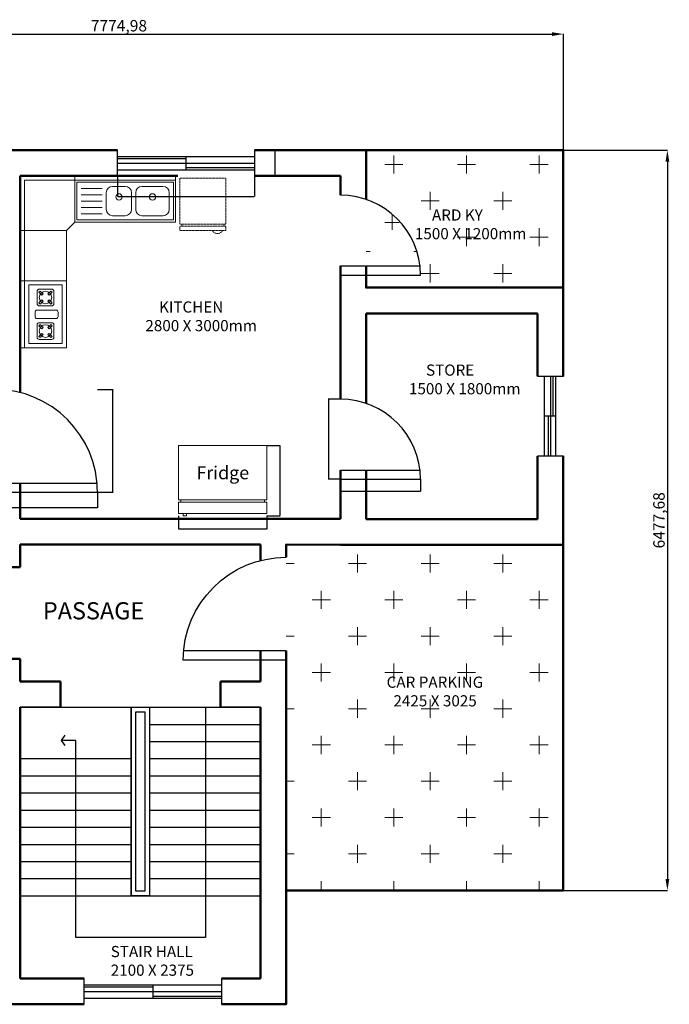
# Model space of a CAD drawing. Units: millimetres. Extents: x -857 to 54106, y -13666 to 13947.
# Tile 12 of 41: x 11637 to 17319, y 5329 to 13947. Entities that reach past the tile are written whole.
import ezdxf

# ---------------------------------------------------------------- set-up
doc = ezdxf.new("R2010")
doc.units = ezdxf.units.MM
doc.linetypes.add('HIDDEN', pattern=[0.375, 0.25, -0.125])
for name, color, linetype, lineweight in [('A-ANNO-DIMS', 2, 'Continuous', 18), ('A-AREA-IDEN', 3, 'Continuous', 18), ('A-DOOR', 1, 'Continuous', 25), ('A-FLOR-FIXT', 8, 'Continuous', 18), ('A-FLOR-FIXT-OVHD', 8, 'HIDDEN', 18), ('A-FLOR-PATT', 252, 'Continuous', 13), ('A-FLOR-STRS', 30, 'Continuous', 25), ('A-GLAZ', 4, 'Continuous', 25), ('A-WALL', 7, 'Continuous', 50), ('FURNITURE', 25, 'Continuous', 9)]:
    doc.layers.add(name, color=color, linetype=linetype, lineweight=lineweight)
doc.styles.add('k.k.', font='arial.ttf')
doc.styles.get("Standard").update_dxf_attribs({"font": 'arial.ttf'})
doc.dimstyles.new('ISO-25', dxfattribs={"dimtxt": 2.5, "dimasz": 2.5, "dimexe": 1.25, "dimexo": 0.625, "dimtad": 1, "dimtxsty": 'Standard', "dimcen": 2.5, "dimadec": 0, "dimazin": 0, "dimtfac": 1, "dimtmove": 0, "dimatfit": 3, "dimfxl": 1, "dimarcsym": 0})

# ---------------------------------------------------------------- blocks, each defined once
blk = doc.blocks.new('A$C338378D9')
at = {"layer": 'FURNITURE'}
for p, q in [((1, -25), (1, -24)), ((38, -25), (38, -24))]:
    blk.add_line(p, q, dxfattribs=at)
for points in [[(0, -24), (39, -24), (39, 0), (0, 0)], [(0, -30), (39, -30), (39, -25), (0, -25)], [(3.5, -31), (2, -31), (2, -30), (3.5, -30)]]:
    blk.add_lwpolyline(points, close=True, dxfattribs=at)
blk = doc.blocks.new('*D25')
at = {"layer": 'A-ANNO-DIMS', "color": 0, "lineweight": -2, "transparency": 16777216}
for p, q in [((8617.3, 12804.9), (8617.3, 13821.5)), ((8717.3, 13820.3), (16292.3, 13820.3)), ((16392.3, 12804.9), (16392.3, 13821.5))]:
    blk.add_line(p, q, dxfattribs=at)
at = {"layer": 'A-ANNO-DIMS', "color": 0, "transparency": 16777216}
for points in [[(8717.3, 13837), (8717.3, 13803.6), (8617.3, 13820.3)], [(16292.3, 13837), (16292.3, 13803.6), (16392.3, 13820.3)]]:
    blk.add_solid(points, dxfattribs=at)
at = {"layer": 'Defpoints', "color": 0, "transparency": 16777216}
for p in [(16392.3, 13820.3), (8617.3, 12804.2), (16392.3, 12804.2)]:
    blk.add_point(p, dxfattribs=at)
at = {"layer": 'A-ANNO-DIMS', "color": 0, "transparency": 16777216, "insert": (12504.8, 13881), "char_height": 100, "attachment_point": 5}
blk.add_mtext('7774,98', dxfattribs=at)
blk = doc.blocks.new('*D26')
at = {"layer": 'A-ANNO-DIMS', "color": 0, "lineweight": -2, "transparency": 16777216}
for p, q in [((16392.9, 12804.2), (17303.8, 12804.2)), ((17302.5, 12704.2), (17302.5, 6426.6)), ((16392.9, 6326.6), (17303.8, 6326.6))]:
    blk.add_line(p, q, dxfattribs=at)
at = {"layer": 'A-ANNO-DIMS', "color": 0, "transparency": 16777216}
for points in [[(17285.9, 12704.2), (17319.2, 12704.2), (17302.5, 12804.2)], [(17285.9, 6426.6), (17319.2, 6426.6), (17302.5, 6326.6)]]:
    blk.add_solid(points, dxfattribs=at)
at = {"layer": 'Defpoints', "color": 0, "transparency": 16777216}
for p in [(16392.3, 12804.2), (16392.3, 6326.6), (17302.5, 6326.6)]:
    blk.add_point(p, dxfattribs=at)
at = {"layer": 'A-ANNO-DIMS', "color": 0, "transparency": 16777216, "insert": (17241.8, 9565.4), "char_height": 100, "attachment_point": 5, "rotation": 90}
blk.add_mtext('6477,68', dxfattribs=at)
blk = doc.blocks.new('DOOR-900')
blk.add_line((11417.3, 9811.5), (12317.3, 9811.5))
blk.add_arc((11417.3, 9811.5), 900, 0, 90)
blk = doc.blocks.new('DOOR-700')
blk.add_line((8245.5, 10779.2), (8245.5, 11479.2))
blk.add_arc((8245.5, 10779.2), 700, 90, 180)
blk = doc.blocks.new('WIN-1200')
for p, q in [((9371.3, 11750.2), (10571.3, 11750.2)), ((9371.3, 11731.7), (9971.3, 11731.7)), ((9971.3, 11750.2), (9971.3, 11630.7)), ((9371.3, 11691.7), (10571.3, 11691.7)), ((9971.3, 11651.7), (10571.3, 11651.7)), ((10571.3, 11630.7), (9371.3, 11630.7))]:
    blk.add_line(p, q)
for points in [[(9371.3, 11579.2), (9371.3, 11804.2)], [(10571.3, 11804.2), (10571.3, 11579.2)]]:
    blk.add_lwpolyline(points)
blk = doc.blocks.new('WIN-700')
for p, q in [((3626.3, 8304.2), (3626.3, 9004.2)), ((3679.8, 9004.2), (3679.8, 8304.2)), ((3699.8, 9004.2), (3699.8, 8654.2)), ((3724.4, 9004.2), (3724.4, 8304.2)), ((3724.4, 8654.2), (3626.3, 8654.2)), ((3659.8, 8654.2), (3659.8, 8304.2))]:
    blk.add_line(p, q)
for points in [[(3567.3, 9004.2), (3792.3, 9004.2)], [(3792.3, 8304.2), (3567.3, 8304.2)]]:
    blk.add_lwpolyline(points)
blk = doc.blocks.new('*D31')
at = {"layer": 'A-ANNO-DIMS', "color": 0, "lineweight": -2, "transparency": 16777216}
for p, q in [((11417.3, 9810.9), (11417.3, 9675.2)), ((12317.3, 9810.9), (12317.3, 9675.2)), ((11419.8, 9676.5), (12314.8, 9676.5))]:
    blk.add_line(p, q, dxfattribs=at)
at = {"layer": 'A-ANNO-DIMS', "color": 0, "transparency": 16777216}
for points in [[(11419.8, 9676.9), (11419.8, 9676.1), (11417.3, 9676.5)], [(12314.8, 9676.9), (12314.8, 9676.1), (12317.3, 9676.5)]]:
    blk.add_solid(points, dxfattribs=at)
at = {"layer": 'Defpoints', "color": 0, "transparency": 16777216}
for p in [(11417.3, 9811.5), (12317.3, 9811.5), (12317.3, 9676.5)]:
    blk.add_point(p, dxfattribs=at)
at = {"layer": 'A-ANNO-DIMS', "color": 0, "transparency": 16777216, "insert": (11867.3, 9678.4), "char_height": 2.5, "attachment_point": 5}
blk.add_mtext('DOOR D1 900 TYP.', dxfattribs=at)
blk = doc.blocks.new('*D32')
at = {"layer": 'A-ANNO-DIMS', "color": 0, "lineweight": -2, "transparency": 16777216}
for p, q in [((12317.9, 10711.5), (12453.5, 10711.5)), ((12452.3, 9814), (12452.3, 10709)), ((12317.9, 9811.5), (12453.5, 9811.5))]:
    blk.add_line(p, q, dxfattribs=at)
at = {"layer": 'A-ANNO-DIMS', "color": 0, "transparency": 16777216}
for points in [[(12451.9, 10709), (12452.7, 10709), (12452.3, 10711.5)], [(12451.9, 9814), (12452.7, 9814), (12452.3, 9811.5)]]:
    blk.add_solid(points, dxfattribs=at)
at = {"layer": 'Defpoints', "color": 0, "transparency": 16777216}
for p in [(12317.3, 10711.5), (12452.3, 10711.5), (12317.3, 9811.5)]:
    blk.add_point(p, dxfattribs=at)
at = {"layer": 'A-ANNO-DIMS', "color": 0, "transparency": 16777216, "insert": (12450.4, 10261.5), "char_height": 2.5, "attachment_point": 5, "rotation": 90}
blk.add_mtext('900 TYP.', dxfattribs=at)
blk = doc.blocks.new('*D33')
at = {"layer": 'A-ANNO-DIMS', "color": 0, "lineweight": -2, "transparency": 16777216}
for p, q in [((14441.7, 10624.9), (14336, 10624.9)), ((14337.3, 10622.4), (14337.3, 9927.4)), ((14441.7, 9924.9), (14336, 9924.9))]:
    blk.add_line(p, q, dxfattribs=at)
at = {"layer": 'A-ANNO-DIMS', "color": 0, "transparency": 16777216}
for points in [[(14336.9, 10622.4), (14337.7, 10622.4), (14337.3, 10624.9)], [(14336.9, 9927.4), (14337.7, 9927.4), (14337.3, 9924.9)]]:
    blk.add_solid(points, dxfattribs=at)
at = {"layer": 'Defpoints', "color": 0, "transparency": 16777216}
for p in [(14442.3, 10624.9), (14337.3, 9924.9), (14442.3, 9924.9)]:
    blk.add_point(p, dxfattribs=at)
at = {"layer": 'A-ANNO-DIMS', "color": 0, "transparency": 16777216, "insert": (14335.4, 10274.9), "char_height": 2.5, "attachment_point": 5, "rotation": 90}
blk.add_mtext('DOOR D2 700 TYP.', dxfattribs=at)
blk = doc.blocks.new('*D34')
at = {"layer": 'A-ANNO-DIMS', "color": 0, "lineweight": -2, "transparency": 16777216}
for p, q in [((14442.3, 9924.3), (14442.3, 9818.7)), ((15142.3, 9924.3), (15142.3, 9818.7)), ((14444.8, 9819.9), (15139.8, 9819.9))]:
    blk.add_line(p, q, dxfattribs=at)
at = {"layer": 'A-ANNO-DIMS', "color": 0, "transparency": 16777216}
for points in [[(14444.8, 9820.4), (14444.8, 9819.5), (14442.3, 9819.9)], [(15139.8, 9820.4), (15139.8, 9819.5), (15142.3, 9819.9)]]:
    blk.add_solid(points, dxfattribs=at)
at = {"layer": 'Defpoints', "color": 0, "transparency": 16777216}
for p in [(14442.3, 9924.9), (15142.3, 9924.9), (15142.3, 9819.9)]:
    blk.add_point(p, dxfattribs=at)
at = {"layer": 'A-ANNO-DIMS', "color": 0, "transparency": 16777216, "insert": (14792.3, 9821.8), "char_height": 2.5, "attachment_point": 5}
blk.add_mtext('700 TYP.', dxfattribs=at)
blk = doc.blocks.new('*D35')
at = {"layer": 'A-ANNO-DIMS', "color": 0, "lineweight": -2, "transparency": 16777216}
for p, q in [((12491.5, 12578.6), (12491.5, 12398)), ((13691.5, 12578.6), (13691.5, 12398)), ((12494, 12399.2), (13689, 12399.2))]:
    blk.add_line(p, q, dxfattribs=at)
at = {"layer": 'A-ANNO-DIMS', "color": 0, "transparency": 16777216}
for points in [[(12494, 12399.6), (12494, 12398.8), (12491.5, 12399.2)], [(13689, 12399.6), (13689, 12398.8), (13691.5, 12399.2)]]:
    blk.add_solid(points, dxfattribs=at)
at = {"layer": 'Defpoints', "color": 0, "transparency": 16777216}
for p in [(12491.5, 12579.2), (13691.5, 12579.2), (13691.5, 12399.2)]:
    blk.add_point(p, dxfattribs=at)
at = {"layer": 'A-ANNO-DIMS', "color": 0, "transparency": 16777216, "insert": (13091.5, 12401.1), "char_height": 2.5, "attachment_point": 5}
blk.add_mtext('WINDOW W1 1200 TYP.', dxfattribs=at)
blk = doc.blocks.new('*D36')
at = {"layer": 'A-ANNO-DIMS', "color": 0, "lineweight": -2, "transparency": 16777216}
for p, q in [((13692.1, 12804.2), (13872.7, 12804.2)), ((13871.5, 12581.7), (13871.5, 12801.7)), ((13692.1, 12579.2), (13872.7, 12579.2))]:
    blk.add_line(p, q, dxfattribs=at)
at = {"layer": 'A-ANNO-DIMS', "color": 0, "transparency": 16777216}
for points in [[(13871.1, 12801.7), (13871.9, 12801.7), (13871.5, 12804.2)], [(13871.1, 12581.7), (13871.9, 12581.7), (13871.5, 12579.2)]]:
    blk.add_solid(points, dxfattribs=at)
at = {"layer": 'Defpoints', "color": 0, "transparency": 16777216}
for p in [(13691.5, 12804.2), (13871.5, 12804.2), (13691.5, 12579.2)]:
    blk.add_point(p, dxfattribs=at)
at = {"layer": 'A-ANNO-DIMS', "color": 0, "transparency": 16777216, "insert": (13869.6, 12691.7), "char_height": 2.5, "attachment_point": 5, "rotation": 90}
blk.add_mtext('225 TYP.', dxfattribs=at)
blk = doc.blocks.new('*D61')
at = {"layer": 'A-ANNO-DIMS', "color": 0, "lineweight": -2, "transparency": 16777216}
for p, q in [((13026.8, 9604.5), (13026.8, 9488)), ((13799.4, 9604.5), (13799.4, 9488)), ((13029.3, 9489.3), (13796.9, 9489.3))]:
    blk.add_line(p, q, dxfattribs=at)
at = {"layer": 'A-ANNO-DIMS', "color": 0, "transparency": 16777216}
for points in [[(13029.3, 9489.7), (13029.3, 9488.8), (13026.8, 9489.3)], [(13796.9, 9489.7), (13796.9, 9488.8), (13799.4, 9489.3)]]:
    blk.add_solid(points, dxfattribs=at)
at = {"layer": 'Defpoints', "color": 0, "transparency": 16777216}
for p in [(13026.8, 9605.1), (13799.4, 9605.1), (13799.4, 9489.3)]:
    blk.add_point(p, dxfattribs=at)
at = {"layer": 'A-ANNO-DIMS', "color": 0, "transparency": 16777216, "insert": (13413.1, 9491.2), "char_height": 2.5, "attachment_point": 5}
blk.add_mtext('FRIDGE 773', dxfattribs=at)
blk = doc.blocks.new('*D62')
at = {"layer": 'A-ANNO-DIMS', "color": 0, "lineweight": -2, "transparency": 16777216}
for p, q in [((13800, 10219.2), (13916.5, 10219.2)), ((13915.3, 9607.6), (13915.3, 10216.7)), ((13800, 9605.1), (13916.5, 9605.1))]:
    blk.add_line(p, q, dxfattribs=at)
at = {"layer": 'A-ANNO-DIMS', "color": 0, "transparency": 16777216}
for points in [[(13914.8, 10216.7), (13915.7, 10216.7), (13915.3, 10219.2)], [(13914.8, 9607.6), (13915.7, 9607.6), (13915.3, 9605.1)]]:
    blk.add_solid(points, dxfattribs=at)
at = {"layer": 'Defpoints', "color": 0, "transparency": 16777216}
for p in [(13799.4, 10219.2), (13915.3, 10219.2), (13799.4, 9605.1)]:
    blk.add_point(p, dxfattribs=at)
at = {"layer": 'A-ANNO-DIMS', "color": 0, "transparency": 16777216, "insert": (13913.3, 9912.2), "char_height": 2.5, "attachment_point": 5, "rotation": 90}
blk.add_mtext('614', dxfattribs=at)

msp = doc.modelspace()

# ---------------------------------------------------------------- hatches: boundary and pattern name
at = {"layer": 'A-FLOR-PATT'}
h = msp.add_hatch(dxfattribs=at)
h.set_pattern_fill('CROSS', color=256, scale=50)
h.set_pattern_definition([(0, (-5489.92, -2561.3), (317.5, 317.5), [158.75, -476.25]), (90, (-5410.54, -2640.7), (-317.5, 317.5), [158.75, -476.25])])
h.paths.add_polyline_path([(16392.264, 9351.555), (14441.85, 9351.555), (13967.28, 9353.369), (13967.28, 9241.901), (13967.28, 8421.901), (13967.28, 6326.555), (16392.264, 6326.555)])
h.paths.add_polyline_path([(16392.264, 12804.231), (14667.264, 12804.231), (14667.264, 12374.147, -0.32131534), (15142.28, 11711.288), (14667.264, 11711.288), (14667.264, 11601.555), (16392.264, 11601.555)])
h.paths.add_polyline_path([(11417.28, 12804.231), (8617.28, 12804.231), (8617.28, 11804.231), (9371.341, 11804.231), (9371.341, 11750.152), (10571.341, 11750.152), (10571.341, 11804.231), (11417.28, 11804.231)])
h = msp.add_hatch(dxfattribs=at)
h.set_pattern_fill('CROSS', color=256, scale=40)
h.set_pattern_definition([(0, (-5489.92, -2561.3), (254, 254), [127, -381]), (90, (-5426.42, -2624.8), (-254, 254), [127, -381])])
h.paths.add_polyline_path([(14667.264, 12374.147), (14667.264, 11791.288), (15137.693, 11791.288, 0.29000459)])

# ---------------------------------------------------------------- linework, layer by layer
at = {"layer": 'A-DOOR'}
for p, q in [((14442.28, 11791.288), (15142.28, 11791.288)), ((14442.28, 10004.935), (15142.28, 10004.935)), ((11417.28, 9891.481), (12317.28, 9891.481)), ((13967.28, 8421.901), (13067.28, 8421.901))]:
    msp.add_line(p, q, dxfattribs=at)
at = {"layer": 'A-FLOR-FIXT'}
for p, q in [((13000.196, 12542.53), (12119.386, 12542.53)), ((12357.938, 12469.13), (12174.436, 12469.13)), ((12357.938, 12414.079), (12174.436, 12414.079)), ((12357.938, 12414.079), (12174.436, 12414.079)), ((12357.938, 12359.028), (12174.436, 12359.028)), ((12357.938, 12303.978), (12174.436, 12303.978)), ((12357.938, 12248.927), (12174.436, 12248.927)), ((11678.98, 12102.125), (11678.98, 11661.72)), ((11678.98, 11661.72), (11678.98, 11074.513))]:
    msp.add_line(p, q, dxfattribs=at)
for points in [[(12119.386, 12175.526), (12119.386, 12579.231), (11642.28, 12579.231), (11642.28, 12102.125), (12045.985, 12102.125)], [(13000.196, 12175.526), (13000.196, 12579.231), (12119.386, 12579.231), (12119.386, 12175.526)], [(12981.846, 12193.876), (12981.846, 12524.18), (12137.736, 12524.18), (12137.736, 12193.876)], [(12045.985, 12102.125), (11642.28, 12102.125), (11642.28, 11661.72), (12045.985, 11661.72)], [(12045.985, 11661.72), (11642.28, 11661.72), (11642.28, 11074.513), (12045.985, 11074.513)], [(12009.284, 11625.019), (11715.681, 11625.019), (11715.681, 11111.213), (12009.284, 11111.213)], [(11831.341, 11535.679), (11805.39, 11561.63), (11815.771, 11572.011), (11841.722, 11546.06)], [(11893.624, 11535.679), (11919.575, 11561.63), (11909.195, 11572.011), (11883.243, 11546.06)], [(11831.341, 11494.157), (11805.39, 11468.206), (11815.771, 11457.826), (11841.722, 11483.777)], [(11893.624, 11494.157), (11919.575, 11468.206), (11909.195, 11457.826), (11883.243, 11483.777)], [(11831.341, 11242.076), (11805.39, 11268.027), (11815.771, 11278.407), (11841.722, 11252.456)], [(11893.624, 11242.076), (11919.575, 11268.027), (11909.195, 11278.407), (11883.243, 11252.456)], [(11831.341, 11200.554), (11805.39, 11174.603), (11815.771, 11164.222), (11841.722, 11190.173)], [(11893.624, 11200.554), (11919.575, 11174.603), (11909.195, 11164.222), (11883.243, 11190.173)]]:
    msp.add_lwpolyline(points, close=True, dxfattribs=at)
msp.add_lwpolyline([(12119.386, 12542.53), (11678.98, 12542.53), (11678.98, 12102.125)], dxfattribs=at)
for points in [[(12559.791, 12487.48, -0.41421356), (12614.842, 12432.429), (12614.842, 12285.627, -0.41421356), (12559.791, 12230.577), (12449.69, 12230.577, -0.41421356), (12394.639, 12285.627), (12394.639, 12432.429, -0.41421356), (12449.69, 12487.48)], [(12890.095, 12487.48, -0.41421356), (12945.145, 12432.429), (12945.145, 12285.627, -0.41421356), (12890.095, 12230.577), (12706.593, 12230.577, -0.41421356), (12651.542, 12285.627), (12651.542, 12432.429, -0.41421356), (12706.593, 12487.48)], [(11935.883, 11459.868), (11935.883, 11569.969, 0.41421356), (11917.533, 11588.319), (11807.432, 11588.319, 0.41421356), (11789.082, 11569.969), (11789.082, 11459.868, 0.41421356), (11807.432, 11441.517), (11917.533, 11441.517, 0.41421356)], [(11972.584, 11349.766), (11972.584, 11386.467, 0.41421356), (11954.234, 11404.817), (11789.082, 11404.817, 0.41421356), (11770.731, 11386.467), (11770.731, 11349.766, 0.41421356), (11789.082, 11331.416), (11954.234, 11331.416, 0.41421356)], [(11935.883, 11276.365), (11935.883, 11166.264, -0.41421356), (11917.533, 11147.914), (11807.432, 11147.914, -0.41421356), (11789.082, 11166.264), (11789.082, 11276.365, -0.41421356), (11807.432, 11294.716), (11917.533, 11294.716, -0.41421356)]]:
    msp.add_lwpolyline(points, format="xyb", close=True, dxfattribs=at)
for centre, radius in [((12504.74, 12395.729), 27.525), ((12798.344, 12395.729), 27.525), ((11862.483, 11514.918), 55.051), ((11862.483, 11221.315), 55.051)]:
    msp.add_circle(centre, radius, dxfattribs=at)
at = {"layer": 'A-FLOR-FIXT-OVHD'}
for p, q in [((13055.247, 12138.826), (13055.247, 12157.176)), ((13422.251, 12138.826), (13422.251, 12157.176)), ((13440.601, 12138.826), (13036.897, 12138.826)), ((13036.897, 12138.826), (13036.897, 12102.125)), ((13036.897, 12102.125), (13440.601, 12102.125)), ((13440.601, 12102.125), (13440.601, 12138.826))]:
    msp.add_line(p, q, dxfattribs=at)
msp.add_lwpolyline([(13440.601, 12560.881), (13440.601, 12157.176), (13036.897, 12157.176), (13036.897, 12560.881)], close=True, dxfattribs=at)
msp.add_arc((13366.68, 12122.628), 48.348, 205.0922551, 334.9077449, dxfattribs=at)
at = {"layer": 'A-FLOR-STRS'}
for p, q in [((11992.28, 7929.231), (11642.28, 7929.231)), ((11642.28, 7929.231), (13742.28, 7929.231)), ((12612.28, 7929.231), (12612.28, 6279.231)), ((12772.28, 7929.231), (12772.28, 6279.231)), ((13742.28, 7929.231), (13392.28, 7929.231)), ((12772.28, 7779.231), (13742.28, 7779.231)), ((12772.28, 7629.231), (13742.28, 7629.231)), ((11642.28, 7479.231), (12612.28, 7479.231)), ((12772.28, 7479.231), (13742.28, 7479.231)), ((11642.28, 7329.231), (12612.28, 7329.231)), ((12772.28, 7329.231), (13742.28, 7329.231)), ((11642.28, 7179.231), (12612.28, 7179.231)), ((12772.28, 7179.231), (13742.28, 7179.231)), ((11642.28, 7029.231), (12612.28, 7029.231)), ((12772.28, 7029.231), (13742.28, 7029.231)), ((11642.28, 6879.231), (12612.28, 6879.231)), ((12772.28, 6879.231), (13742.28, 6879.231)), ((11642.28, 6729.231), (12612.28, 6729.231)), ((12772.28, 6729.231), (13742.28, 6729.231)), ((11642.28, 6579.231), (12612.28, 6579.231)), ((12772.28, 6579.231), (13742.28, 6579.231)), ((11642.28, 6429.231), (12612.28, 6429.231)), ((12772.28, 6429.231), (13742.28, 6429.231)), ((11642.28, 6279.231), (13742.28, 6279.231))]:
    msp.add_line(p, q, dxfattribs=at)
for points in [[(13263.236, 7929.231), (13263.236, 5914.255), (12127.28, 5914.255), (12127.28, 7637.854), (12000.518, 7637.854)], [(12031.972, 7684.139), (12000.518, 7637.854), (12030.82, 7594.913)]]:
    msp.add_lwpolyline(points, dxfattribs=at)
for points in [[(12612.28, 7929.231), (12772.28, 7929.231), (12772.28, 6279.231), (12612.28, 6279.231)], [(12652.28, 7889.231), (12732.28, 7889.231), (12732.28, 6319.231), (12652.28, 6319.231)]]:
    msp.add_lwpolyline(points, close=True, dxfattribs=at)
at = {"layer": 'A-WALL'}
for p, q in [((11642.28, 12804.231), (12491.498, 12804.231)), ((13691.498, 12804.231), (14667.264, 12804.231)), ((11642.28, 12579.231), (13020.052, 12579.231)), ((11642.28, 10682.903), (11642.28, 12579.231)), ((13691.498, 12579.231), (14442.28, 12579.231)), ((14442.28, 12579.231), (14442.28, 12411.288)), ((14442.28, 12579.231), (14442.28, 12411.288)), ((14442.28, 11791.288), (14442.28, 11380.304)), ((14442.28, 11791.288), (14442.28, 10624.935)), ((14667.264, 11376.555), (16167.264, 11376.555)), ((14667.264, 10587.794), (14667.264, 11376.555)), ((16167.264, 11376.555), (16167.264, 10826.555)), ((16167.264, 10126.555), (16167.264, 9576.555)), ((14442.28, 10004.935), (14442.28, 9579.231)), ((14667.264, 9576.555), (14667.264, 10004.935)), ((11642.28, 9579.231), (11642.28, 9891.481)), ((14442.28, 9579.231), (11642.28, 9579.231)), ((16167.264, 9576.555), (14667.264, 9576.555)), ((13742.28, 9354.231), (11642.28, 9354.231)), ((11642.28, 9354.231), (11642.28, 9154.231)), ((13742.28, 9213.322), (13742.28, 9354.231)), ((16392.264, 9351.555), (16392.264, 6326.555)), ((11642.28, 9154.231), (11417.28, 9154.231)), ((13742.28, 8154.231), (13742.28, 8421.901)), ((11642.28, 8354.231), (11417.28, 8354.231)), ((11642.28, 8354.231), (11642.28, 8154.231)), ((11642.28, 8154.231), (11992.28, 8154.231)), ((11992.28, 8154.231), (11992.28, 7929.231)), ((13392.28, 7929.231), (13392.28, 8154.231)), ((13392.28, 8154.231), (13742.28, 8154.231)), ((11642.28, 5554.231), (11642.28, 7929.231)), ((13742.28, 7929.231), (13742.28, 5554.231)), ((16392.264, 6326.555), (13967.28, 6326.555)), ((12200.793, 5554.231), (11642.28, 5554.231)), ((12200.793, 5554.231), (11642.28, 5554.231)), ((13742.28, 5554.231), (13400.793, 5554.231)), ((13742.28, 5554.231), (13400.793, 5554.231))]:
    msp.add_line(p, q, dxfattribs=at)
for points in [[(10571.341, 11804.231), (11417.28, 11804.231), (11417.28, 12804.231), (11642.28, 12804.231)], [(14667.264, 12804.231), (14667.264, 12374.147)], [(14667.264, 11791.288), (14667.264, 11601.555), (16392.264, 11601.555), (16392.264, 12804.231), (14667.264, 12804.231), (14667.264, 12374.147)], [(14667.264, 11791.288), (14667.264, 11601.555), (16392.264, 11601.555), (16392.264, 10826.555)], [(16392.264, 10126.555), (16392.264, 9351.555), (14441.85, 9351.555), (13967.28, 9353.369), (13967.28, 9241.901)], [(13967.28, 8421.901), (13967.28, 5329.231), (13400.793, 5329.231)], [(12200.793, 5329.231), (11263.585, 5329.231)]]:
    msp.add_lwpolyline(points, dxfattribs=at)

# ---------------------------------------------------------------- block references
at = {"layer": 'A-DOOR'}
for p, rotation in [((3663.049, 19956.834), 269.9999999999999), ((3663.049, 18170.481), 270)]:
    msp.add_blockref('DOOR-700', p, dxfattribs=dict(at, rotation=rotation))
msp.add_blockref('DOOR-900', (0, 0), dxfattribs=at)
at = {"layer": 'A-DOOR', "extrusion": (0, 0, -1), "zscale": -1}
msp.add_blockref('DOOR-900', (-25384.56, -1469.581), dxfattribs=at)
at = {"layer": 'A-FLOR-FIXT', "xscale": 19.80925460289891, "yscale": 19.80925460289891, "zscale": 19.80925460289891}
msp.add_blockref('A$C338378D9', (13026.805, 10219.222), dxfattribs=at)
at = {"layer": 'A-GLAZ'}
for name, p in [('WIN-1200', (3120.157, 1000)), ('WIN-700', (12599.984, 1822.324)), ('WIN-1200', (2829.453, -6250))]:
    msp.add_blockref(name, p, dxfattribs=at)

# ---------------------------------------------------------------- texts
at = {"layer": 'A-AREA-IDEN', "attachment_point": 1}
for s, width, gutter_width, heights, insert, char_height in [('\\pxt0;     ARD KY\\P1500 X 1200mm', 2554.22693, 18810.576, [2595.835], (15093.908, 12285.937), 97.80511), ('\\pxt0;    KITCHEN\\P2800 X 3000mm', 1660.07971, 12225.639, [1687.122], (12736.18, 11480.988), 97.80511), ('\\pxt0;     STORE\\P1500 X 1800mm', 2554.22693, 18810.576, [2595.835], (15042.007, 10928.71), 97.80511), ('\\pxt0;PASSAGE', 2554.22693, 18810.576, [2595.835], (11839.321, 8848.577), 150.48461), ('\\pxt0;CAR PARKING\\P  2425 X 3025', 2554.22693, 18810.576, [2595.835], (14846.419, 8197.383), 97.80511), ('\\pxt0;STAIR HALL\\P2100 X 2375', 2554.22693, 18810.576, [2595.835], (12433.119, 5839.865), 97.80511)]:
    msp.add_mtext_dynamic_manual_height_columns(s, width=width, gutter_width=gutter_width, heights=heights, dxfattribs=dict(at, insert=insert, char_height=char_height))
at = {"layer": 'A-AREA-IDEN', "insert": (13413.086, 9981.511), "char_height": 114.4535, "attachment_point": 5, "style": 'k.k.'}
msp.add_mtext_dynamic_manual_height_columns('\\A1;Fridge', width=476.30239, gutter_width=858.401, heights=[0], dxfattribs=at)

# ---------------------------------------------------------------- dimensions: what is measured, and where the dimension line sits
at = {"layer": 'A-ANNO-DIMS'}
dim = msp.add_linear_dim(base=(16392.264, 13820.288), p1=(8617.28, 12804.231), p2=(16392.264, 12804.231), dimstyle='ISO-25', override={"dimtxt": 100, "dimasz": 100, "dimclrd": 0, "dimclre": 0, "dimclrt": 0}, dxfattribs=at)
dim.commit()
dim.dimension.update_dxf_attribs({"geometry": '*D25', "text_midpoint": (12504.772, 13881.008)})
for base, p1, p2, angle, text, picture, middle in [((13871.498, 12804.231), (13691.498, 12579.231), (13691.498, 12804.231), 90, '<> TYP.', '*D36', (13869.597, 12691.731)), ((12452.28, 10711.481), (12317.28, 9811.481), (12317.28, 10711.481), 90, '<> TYP.', '*D32', (12450.379, 10261.481)), ((14337.28, 9924.935), (14442.28, 10624.935), (14442.28, 9924.935), 270, 'DOOR D2 <> TYP.', '*D33', (14335.361, 10274.935))]:
    dim = msp.add_linear_dim(base=base, p1=p1, p2=p2, angle=angle, text=text, dimstyle='ISO-25', override={"dimdec": 0, "dimrnd": 0, "dimzin": 0, "dimlunit": 2}, dxfattribs=at)
    dim.commit()
    dim.dimension.update_dxf_attribs({"geometry": picture, "text_midpoint": middle})
for base, p1, p2, override, picture, middle in [((17302.536, 6326.555), (16392.264, 12804.231), (16392.264, 6326.555), {"dimtxt": 100, "dimasz": 100, "dimclrd": 0, "dimclre": 0, "dimclrt": 0}, '*D26', (17241.815, 9565.393)), ((13915.25, 10219.222), (13799.366, 9605.135), (13799.366, 10219.222), {"dimdec": 0, "dimrnd": 0, "dimzin": 0, "dimlunit": 2}, '*D62', (13913.349, 9912.178))]:
    dim = msp.add_linear_dim(base=base, p1=p1, p2=p2, angle=90, dimstyle='ISO-25', override=override, dxfattribs=at)
    dim.commit()
    dim.dimension.update_dxf_attribs({"geometry": picture, "text_midpoint": middle})
for base, p1, p2, text, picture, middle in [((13691.498, 12399.231), (12491.498, 12579.231), (13691.498, 12579.231), 'WINDOW W1 <> TYP.', '*D35', (13091.498, 12401.149)), ((15142.28, 9819.935), (14442.28, 9924.935), (15142.28, 9924.935), '<> TYP.', '*D34', (14792.28, 9821.837)), ((12317.28, 9676.481), (11417.28, 9811.481), (12317.28, 9811.481), 'DOOR D1 <> TYP.', '*D31', (11867.28, 9678.4)), ((13799.366, 9489.251), (13026.805, 9605.135), (13799.366, 9605.135), 'FRIDGE <>', '*D61', (13413.086, 9491.169))]:
    dim = msp.add_linear_dim(base=base, p1=p1, p2=p2, text=text, dimstyle='ISO-25', override={"dimdec": 0, "dimrnd": 0, "dimzin": 0, "dimlunit": 2}, dxfattribs=at)
    dim.commit()
    dim.dimension.update_dxf_attribs({"geometry": picture, "text_midpoint": middle})

doc.saveas('drawing.dxf')
